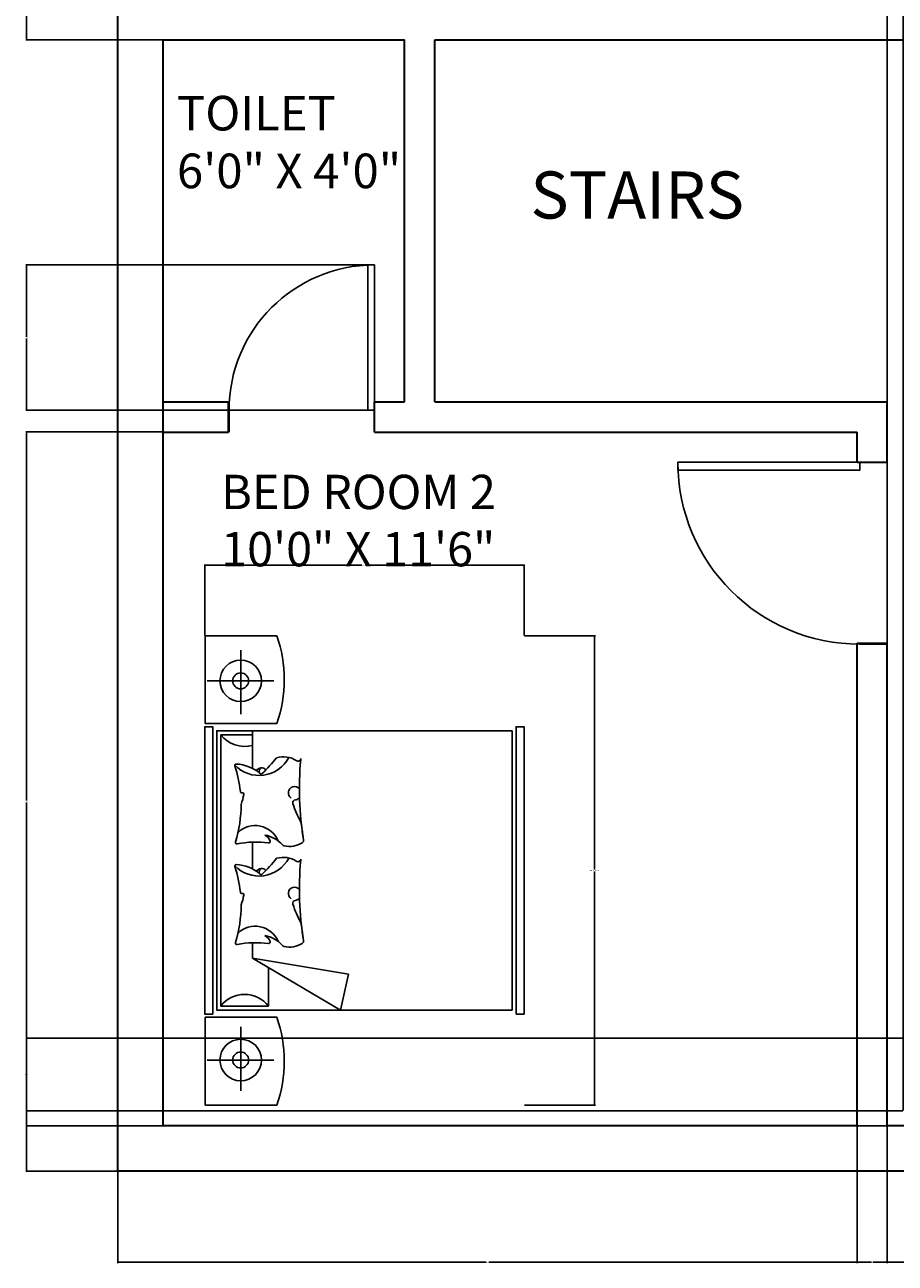
# Model space of a CAD drawing. Units: inches. Extents: x 2360 to 2721, y 1697 to 2094.
# Tile 1 of 3: x 2360 to 2533, y 1697 to 1944. Entities that reach past the tile are written whole.
import ezdxf

# ---------------------------------------------------------------- set-up
doc = ezdxf.new("R2010")
doc.units = ezdxf.units.IN
for name, color, linetype, lineweight in [('A-ANNO-DIMS', 2, 'Continuous', 18), ('A-AREA-IDEN', 7, 'Continuous', 18), ('A-DOOR', 4, 'Continuous', 25), ('A-WALL', 7, 'Continuous', 35), ('FUR', 42, 'Continuous', 18)]:
    doc.layers.add(name, color=color, linetype=linetype, lineweight=lineweight)
for name, color, linetype in [('HID', 11, 'Continuous'), ('SAN', 5, 'Continuous'), ('wood', 26, 'Continuous')]:
    doc.layers.add(name, color=color, linetype=linetype)
doc.styles.get("Standard").update_dxf_attribs({"font": 'arial.ttf'})
doc.dimstyles.get("Standard").update_dxf_attribs({"dimtxt": 0.18, "dimasz": 0.18, "dimexe": 0.18, "dimexo": 0.0625, "dimgap": 0.09, "dimtad": 0, "dimtih": 1, "dimtoh": 1, "dimdec": 4, "dimzin": 0, "dimdsep": 46, "dimtxsty": 'Standard', "dimcen": 0.09, "dimadec": 0, "dimazin": 0, "dimtfac": 1, "dimtdec": 4, "dimtofl": 0, "dimtmove": 0, "dimatfit": 3, "dimfxl": 1, "dimtolj": 1, "dimtzin": 0, "dimarcsym": 0})

# ---------------------------------------------------------------- blocks, each defined once
blk = doc.blocks.new('*U2')
for p, q in [((0, 0), (0, -6)), ((-40, 0), (-40, -6))]:
    blk.add_line(p, q)
blk.add_lwpolyline([(0, 0), (0, 40), (-1.75, 40), (-1.75, 0)], close=True)
blk.add_arc((0, 0), 40, 90, 180)
blk = doc.blocks.new('A$C47AC156F')
at = {"layer": 'HID'}
for centre, radius, start, end in [((1.0153, 1.7986), 0.00933, 72.72477, 190.95899), ((0.3959, 1.6787), 0.6216, 352.73629, 10.95899), ((1.25, 2.5533), 0.781, 252.72477, 270.27016), ((0.9655, 1.684), 0.1552, 292.76276, 43.89219), ((1.25, 2.5533), 0.781, 276.21957, 288.21138), ((1.6451, 1.66), 0.2103, 133.89466, 242.39517), ((1.258, 1.8145), 0.2487, 319.92106, 357.12402), ((1.497, 1.8025), 0.00933, 357.12402, 108.21138), ((1.497, 1.8025), 0.00933, 357.12402, 108.21138), ((1.6455, 1.7986), 0.00933, 72.72477, 190.95899), ((1.0261, 1.6787), 0.6216, 352.73629, 10.95899), ((1.8802, 2.5533), 0.781, 252.72477, 270.27016), ((1.5957, 1.684), 0.1552, 292.76276, 43.89219), ((1.8802, 2.5533), 0.781, 276.21957, 288.21138), ((2.2753, 1.66), 0.2103, 133.89466, 242.39517), ((1.8881, 1.8145), 0.2487, 319.92106, 357.12402), ((2.1272, 1.8025), 0.00933, 357.12402, 108.21138), ((2.1272, 1.8025), 0.00933, 357.12402, 108.21138), ((1.3847, 2.1211), 0.3726, 249.41677, 259.30852), ((1.3173, 1.7641), 0.00933, 259.30852, 10.68903), ((1.3356, 1.7676), 0.00933, 96.21957, 190.68903), ((2.0148, 2.1211), 0.3726, 249.41677, 259.30852), ((1.9474, 1.7641), 0.00933, 259.30852, 10.68903), ((1.9658, 1.7676), 0.00933, 96.21957, 190.68903), ((1.4528, 1.6463), 0.00933, 118.83153, 225.83293), ((2.7269, 2.958), 1.838, 225.83293, 230.02451), ((0.9938, -0.376), 2.0876, 76.49824, 77.28883), ((1.4453, 1.6438), 0.0373, 312.66199, 59.15728), ((2.0829, 1.6463), 0.00933, 118.83153, 225.83293), ((3.357, 2.958), 1.838, 225.83293, 230.02451), ((1.6239, -0.376), 2.0876, 76.49824, 77.28883), ((2.0754, 1.6438), 0.0373, 312.66199, 59.15728), ((0.8707, 1.6576), 0.1939, 311.60711, 349.78448), ((1.0218, 1.5989), 0.00933, 172.73629, 288.29854), ((1.0054, 1.6485), 0.0615, 288.29854, 335.78909), ((0.9938, 3.6438), 2.0876, 282.70178, 282.72062), ((1.5008, 1.6576), 0.1939, 311.60711, 349.78448), ((1.6519, 1.5989), 0.00933, 172.73629, 288.29854), ((1.6355, 1.6485), 0.0615, 288.29854, 335.78909), ((1.6239, 3.6438), 2.0876, 282.70178, 282.72062), ((1.1421, 1.4694), 0.1522, 167.33771, 211.66603), ((1.0118, 1.4987), 0.0187, 131.60711, 167.33771), ((1.3258, 1.4364), 0.0395, 312.35651, 145.77621), ((1.4005, 1.5084), 0.1512, 327.16626, 15.7613), ((1.7723, 1.4694), 0.1522, 167.33771, 211.66603), ((1.642, 1.4987), 0.0187, 131.60711, 167.33771), ((1.9559, 1.4364), 0.0395, 312.35651, 145.77621), ((2.0307, 1.5084), 0.1512, 327.16626, 15.7613), ((1.3501, -0.5337), 1.9409, 84.58522, 99.44651), ((1.1321, 1.4137), 0.0187, 276.38601, 303.79553), ((1.5399, 0.631), 0.864, 109.04896, 117.38232), ((1.264, 1.43), 0.0187, 2.64257, 109.04896), ((1.3013, 1.4318), 0.0187, 182.64257, 192.70152), ((1.3234, 1.4368), 0.0414, 192.70152, 227.15561), ((1.5433, 1.4163), 0.0187, 147.16626, 264.34216), ((1.9802, -0.5337), 1.9409, 84.58522, 99.44651), ((1.7622, 1.4137), 0.0187, 276.38601, 303.79553), ((2.17, 0.631), 0.864, 109.04896, 117.38232), ((1.8941, 1.43), 0.0187, 2.64257, 109.04896), ((1.9314, 1.4318), 0.0187, 182.64257, 192.70152), ((1.9535, 1.4368), 0.0414, 192.70152, 227.15561), ((2.1734, 1.4163), 0.0187, 147.16626, 264.34216), ((1.0285, 1.3993), 0.0187, 211.66603, 279.44651), ((1.3501, -0.5337), 1.9409, 96.38601, 99.44651), ((1.6586, 1.3993), 0.0187, 211.66603, 279.44651), ((1.9802, -0.5337), 1.9409, 96.38601, 99.44651)]:
    blk.add_arc(centre, radius, start, end, dxfattribs=at)
at = {"layer": 'SAN'}
for p, q in [((0.2826, 1.9847), (0.2826, 1.5664)), ((2.6574, 1.9847), (2.6574, 1.5664)), ((0.0902, 1.7748), (0.4911, 1.7748)), ((2.8498, 1.7748), (2.4489, 1.7748))]:
    blk.add_line(p, q, dxfattribs=at)
for centre, radius in [((0.2826, 1.7748), 0.13), ((2.6574, 1.7748), 0.13), ((0.2826, 1.7748), 0.05), ((2.6574, 1.7748), 0.05)]:
    blk.add_circle(centre, radius, dxfattribs=at)
at = {"layer": 'wood'}
for p, q in [((0, 1.9982), (0, 1.5482)), ((0.55, 1.9982), (0, 1.9982)), ((0.55, 1.9982), (0.55, 1.5482)), ((2.39, 1.9982), (2.94, 1.9982)), ((2.39, 1.9982), (2.39, 1.5482)), ((2.94, 1.9982), (2.94, 1.5482)), ((0.62, 1.9), (2.32, 1.9)), ((0.62, 1.9), (0.62, 1.6)), ((2.32, 1.9), (2.32, 1.7)), ((0.92, 1.7), (0.595, 1.15)), ((0.82, 1.1), (0.92, 1.7)), ((1.0171, 1.7), (0.92, 1.7)), ((1.6473, 1.7), (1.4787, 1.7)), ((2.345, 1.7), (2.1088, 1.7)), ((0.62, 1.6), (0.8609, 1.6)), ((0.595, 1.15), (0.82, 1.1))]:
    blk.add_line(p, q, dxfattribs=at)
for points in [[(0.57, 1.95), (2.37, 1.95), (2.37, 2), (0.57, 2)], [(2.345, 0.075), (2.345, 1.925), (0.595, 1.925), (0.595, 0.075)], [(0.57, 0.05), (2.37, 0.05), (2.37, 0), (0.57, 0)]]:
    blk.add_lwpolyline(points, close=True, dxfattribs=at)
for centre, radius, start, end in [((0.5037, 1.75), 0.1898, 307.78263, 52.21737), ((2.4363, 1.75), 0.1898, 127.78263, 195.27469), ((0.275, 2.3419), 0.84, 250.89004, 289.10996), ((2.665, 2.3419), 0.84, 250.89004, 289.10996)]:
    blk.add_arc(centre, radius, start, end, dxfattribs=at)
blk = doc.blocks.new('*D9')
at = {"layer": 'A-ANNO-DIMS', "color": 0, "lineweight": -2, "transparency": 16777216}
for p, q in [((2459.47, 1822.13), (2473.59, 1822.13)), ((2473.41, 1821.95), (2473.41, 1775.63)), ((2473.41, 1728.94), (2473.41, 1775.26)), ((2459.47, 1728.76), (2473.59, 1728.76))]:
    blk.add_line(p, q, dxfattribs=at)
at = {"layer": 'A-ANNO-DIMS', "color": 0, "transparency": 16777216}
for points in [[(2473.38, 1821.95), (2473.44, 1821.95), (2473.41, 1822.13)], [(2473.38, 1728.94), (2473.44, 1728.94), (2473.41, 1728.76)]]:
    blk.add_solid(points, dxfattribs=at)
at = {"layer": 'Defpoints', "color": 0, "transparency": 16777216}
for p in [(2459.41, 1822.13), (2473.41, 1822.13), (2459.41, 1728.76)]:
    blk.add_point(p, dxfattribs=at)
at = {"layer": 'A-ANNO-DIMS', "color": 0, "transparency": 16777216, "insert": (2473.41, 1775.44), "char_height": 0.18, "attachment_point": 5}
blk.add_mtext('\\A1;BED SET 93 TYP.', dxfattribs=at)
blk = doc.blocks.new('*D10')
at = {"layer": 'A-ANNO-DIMS', "color": 0, "lineweight": -2, "transparency": 16777216}
for p, q in [((2395.9, 1822.19), (2395.9, 1836.31)), ((2396.08, 1836.13), (2427.13, 1836.13)), ((2459.23, 1836.13), (2428.18, 1836.13)), ((2459.41, 1822.19), (2459.41, 1836.31))]:
    blk.add_line(p, q, dxfattribs=at)
at = {"layer": 'A-ANNO-DIMS', "color": 0, "transparency": 16777216}
for points in [[(2396.08, 1836.16), (2396.08, 1836.1), (2395.9, 1836.13)], [(2459.23, 1836.16), (2459.23, 1836.1), (2459.41, 1836.13)]]:
    blk.add_solid(points, dxfattribs=at)
at = {"layer": 'Defpoints', "color": 0, "transparency": 16777216}
for p in [(2395.9, 1836.13), (2395.9, 1822.13), (2459.41, 1822.13)]:
    blk.add_point(p, dxfattribs=at)
at = {"layer": 'A-ANNO-DIMS', "color": 0, "transparency": 16777216, "insert": (2427.65, 1836.13), "char_height": 0.18, "attachment_point": 5}
blk.add_mtext('\\A1;64 TYP.', dxfattribs=at)
blk = doc.blocks.new('*D19')
at = {"layer": 'A-ANNO-DIMS', "color": 0, "lineweight": -2, "transparency": 16777216}
for p, q in [((2525.63, 1724.58), (2525.63, 1697.32)), ((2378.63, 1715.58), (2378.63, 1697.32)), ((2378.81, 1697.5), (2451.85, 1697.5)), ((2525.45, 1697.5), (2452.41, 1697.5))]:
    blk.add_line(p, q, dxfattribs=at)
at = {"layer": 'A-ANNO-DIMS', "color": 0, "transparency": 16777216}
for points in [[(2378.81, 1697.53), (2378.81, 1697.47), (2378.63, 1697.5)], [(2525.45, 1697.53), (2525.45, 1697.47), (2525.63, 1697.5)]]:
    blk.add_solid(points, dxfattribs=at)
at = {"layer": 'Defpoints', "color": 0, "transparency": 16777216}
for p in [(2525.63, 1724.65), (2378.63, 1715.65), (2525.63, 1697.5)]:
    blk.add_point(p, dxfattribs=at)
at = {"layer": 'A-ANNO-DIMS', "color": 0, "transparency": 16777216, "insert": (2452.13, 1697.5), "char_height": 0.18, "attachment_point": 5}
blk.add_mtext('\\A1;147', dxfattribs=at)
blk = doc.blocks.new('*D20')
at = {"layer": 'A-ANNO-DIMS', "color": 0, "lineweight": -2, "transparency": 16777216}
for p, q in [((2525.63, 1724.58), (2525.63, 1697.32)), ((2531.63, 1724.58), (2531.63, 1697.32)), ((2525.81, 1697.5), (2528.48, 1697.5)), ((2531.45, 1697.5), (2528.78, 1697.5))]:
    blk.add_line(p, q, dxfattribs=at)
at = {"layer": 'A-ANNO-DIMS', "color": 0, "transparency": 16777216}
for points in [[(2525.81, 1697.53), (2525.81, 1697.47), (2525.63, 1697.5)], [(2531.45, 1697.53), (2531.45, 1697.47), (2531.63, 1697.5)]]:
    blk.add_solid(points, dxfattribs=at)
at = {"layer": 'Defpoints', "color": 0, "transparency": 16777216}
for p in [(2525.63, 1724.65), (2531.63, 1724.65), (2531.63, 1697.5)]:
    blk.add_point(p, dxfattribs=at)
at = {"layer": 'A-ANNO-DIMS', "color": 0, "transparency": 16777216, "insert": (2528.63, 1697.5), "char_height": 0.18, "attachment_point": 5}
blk.add_mtext('\\A1;6', dxfattribs=at)
blk = doc.blocks.new('*D21')
at = {"layer": 'A-ANNO-DIMS', "color": 0, "lineweight": -2, "transparency": 16777216}
for p, q in [((2531.63, 1724.58), (2531.63, 1697.32)), ((2609.63, 1724.58), (2609.63, 1697.32)), ((2531.81, 1697.5), (2570.41, 1697.5)), ((2609.45, 1697.5), (2570.85, 1697.5))]:
    blk.add_line(p, q, dxfattribs=at)
at = {"layer": 'A-ANNO-DIMS', "color": 0, "transparency": 16777216}
for points in [[(2531.81, 1697.53), (2531.81, 1697.47), (2531.63, 1697.5)], [(2609.45, 1697.53), (2609.45, 1697.47), (2609.63, 1697.5)]]:
    blk.add_solid(points, dxfattribs=at)
at = {"layer": 'Defpoints', "color": 0, "transparency": 16777216}
for p in [(2531.63, 1724.65), (2609.63, 1724.65), (2609.63, 1697.5)]:
    blk.add_point(p, dxfattribs=at)
at = {"layer": 'A-ANNO-DIMS', "color": 0, "transparency": 16777216, "insert": (2570.63, 1697.5), "char_height": 0.18, "attachment_point": 5}
blk.add_mtext('\\A1;78', dxfattribs=at)
blk = doc.blocks.new('*D24')
at = {"layer": 'A-ANNO-DIMS', "color": 0, "lineweight": -2, "transparency": 16777216}
for p, q in [((2387.57, 1862.65), (2360.3, 1862.65)), ((2360.48, 1862.47), (2360.48, 1789.33)), ((2360.48, 1715.83), (2360.48, 1788.97)), ((2378.57, 1715.65), (2360.3, 1715.65))]:
    blk.add_line(p, q, dxfattribs=at)
at = {"layer": 'A-ANNO-DIMS', "color": 0, "transparency": 16777216}
for points in [[(2360.45, 1862.47), (2360.51, 1862.47), (2360.48, 1862.65)], [(2360.45, 1715.83), (2360.51, 1715.83), (2360.48, 1715.65)]]:
    blk.add_solid(points, dxfattribs=at)
at = {"layer": 'Defpoints', "color": 0, "transparency": 16777216}
for p in [(2360.48, 1862.65), (2387.63, 1862.65), (2378.63, 1715.65)]:
    blk.add_point(p, dxfattribs=at)
at = {"layer": 'A-ANNO-DIMS', "color": 0, "transparency": 16777216, "insert": (2360.48, 1789.15), "char_height": 0.18, "attachment_point": 5}
blk.add_mtext('\\A1;147', dxfattribs=at)
blk = doc.blocks.new('*D25')
at = {"layer": 'A-ANNO-DIMS', "color": 0, "lineweight": -2, "transparency": 16777216}
for p, q in [((2429.57, 1895.87), (2360.3, 1895.87)), ((2360.48, 1895.69), (2360.48, 1881.61)), ((2360.48, 1867.16), (2360.48, 1881.24)), ((2429.57, 1866.98), (2360.3, 1866.98))]:
    blk.add_line(p, q, dxfattribs=at)
at = {"layer": 'A-ANNO-DIMS', "color": 0, "transparency": 16777216}
for points in [[(2360.45, 1895.69), (2360.51, 1895.69), (2360.48, 1895.87)], [(2360.45, 1867.16), (2360.51, 1867.16), (2360.48, 1866.98)]]:
    blk.add_solid(points, dxfattribs=at)
at = {"layer": 'Defpoints', "color": 0, "transparency": 16777216}
for p in [(2360.48, 1895.87), (2429.63, 1895.87), (2429.63, 1866.98)]:
    blk.add_point(p, dxfattribs=at)
at = {"layer": 'A-ANNO-DIMS', "color": 0, "transparency": 16777216, "insert": (2360.48, 1881.43), "char_height": 0.18, "attachment_point": 5}
blk.add_mtext('\\A1;28.89', dxfattribs=at)
blk = doc.blocks.new('*D26')
at = {"layer": 'A-ANNO-DIMS', "color": 0, "lineweight": -2, "transparency": 16777216}
for p, q in [((2387.57, 1976.65), (2360.3, 1976.65)), ((2360.48, 1976.47), (2360.48, 1958.83)), ((2360.48, 1940.83), (2360.48, 1958.46)), ((2387.57, 1940.65), (2360.3, 1940.65))]:
    blk.add_line(p, q, dxfattribs=at)
at = {"layer": 'A-ANNO-DIMS', "color": 0, "transparency": 16777216}
for points in [[(2360.45, 1976.47), (2360.51, 1976.47), (2360.48, 1976.65)], [(2360.45, 1940.83), (2360.51, 1940.83), (2360.48, 1940.65)]]:
    blk.add_solid(points, dxfattribs=at)
at = {"layer": 'Defpoints', "color": 0, "transparency": 16777216}
for p in [(2360.48, 1976.65), (2387.63, 1976.65), (2387.63, 1940.65)]:
    blk.add_point(p, dxfattribs=at)
at = {"layer": 'A-ANNO-DIMS', "color": 0, "transparency": 16777216, "insert": (2360.48, 1958.65), "char_height": 0.18, "attachment_point": 5}
blk.add_mtext('\\A1;36', dxfattribs=at)
blk = doc.blocks.new('*D36')
at = {"layer": 'A-ANNO-DIMS', "color": 0, "lineweight": -2, "transparency": 16777216}
for p, q in [((2544.4, 1742.08), (2360.3, 1742.08)), ((2360.48, 1741.9), (2360.48, 1735.04)), ((2360.48, 1727.81), (2360.48, 1734.67)), ((2534.77, 1727.63), (2360.3, 1727.63))]:
    blk.add_line(p, q, dxfattribs=at)
at = {"layer": 'A-ANNO-DIMS', "color": 0, "transparency": 16777216}
for points in [[(2360.45, 1741.9), (2360.51, 1741.9), (2360.48, 1742.08)], [(2360.45, 1727.81), (2360.51, 1727.81), (2360.48, 1727.63)]]:
    blk.add_solid(points, dxfattribs=at)
at = {"layer": 'Defpoints', "color": 0, "transparency": 16777216}
for p in [(2360.48, 1742.08), (2544.47, 1742.08), (2534.83, 1727.63)]:
    blk.add_point(p, dxfattribs=at)
at = {"layer": 'A-ANNO-DIMS', "color": 0, "transparency": 16777216, "insert": (2360.48, 1734.85), "char_height": 0.18, "attachment_point": 5}
blk.add_mtext('\\A1;14.454', dxfattribs=at)
blk = doc.blocks.new('*D37')
at = {"layer": 'A-ANNO-DIMS', "color": 0, "lineweight": -2, "transparency": 16777216}
for p, q in [((2531.63, 1724.71), (2531.63, 2093.98)), ((2534.83, 1727.69), (2534.83, 2093.98)), ((2531.81, 2093.8), (2532.84, 2093.8)), ((2534.65, 2093.8), (2533.63, 2093.8))]:
    blk.add_line(p, q, dxfattribs=at)
at = {"layer": 'A-ANNO-DIMS', "color": 0, "transparency": 16777216}
for points in [[(2531.81, 2093.83), (2531.81, 2093.77), (2531.63, 2093.8)], [(2534.65, 2093.83), (2534.65, 2093.77), (2534.83, 2093.8)]]:
    blk.add_solid(points, dxfattribs=at)
at = {"layer": 'Defpoints', "color": 0, "transparency": 16777216}
for p in [(2534.83, 2093.8), (2534.83, 1727.63), (2531.63, 1724.65)]:
    blk.add_point(p, dxfattribs=at)
at = {"layer": 'A-ANNO-DIMS', "color": 0, "transparency": 16777216, "insert": (2533.23, 2093.8), "char_height": 0.18, "attachment_point": 5}
blk.add_mtext('\\A1;3.198', dxfattribs=at)
blk = doc.blocks.new('*D38')
at = {"layer": 'A-ANNO-DIMS', "color": 0, "lineweight": -2, "transparency": 16777216}
for p, q in [((2534.77, 1727.63), (2360.3, 1727.63)), ((2360.48, 1727.45), (2360.48, 1726.32)), ((2531.57, 1724.65), (2360.3, 1724.65)), ((2360.48, 1724.83), (2360.48, 1725.95))]:
    blk.add_line(p, q, dxfattribs=at)
at = {"layer": 'A-ANNO-DIMS', "color": 0, "transparency": 16777216}
for points in [[(2360.45, 1727.45), (2360.51, 1727.45), (2360.48, 1727.63)], [(2360.45, 1724.83), (2360.51, 1724.83), (2360.48, 1724.65)]]:
    blk.add_solid(points, dxfattribs=at)
at = {"layer": 'Defpoints', "color": 0, "transparency": 16777216}
for p in [(2360.48, 1727.63), (2534.83, 1727.63), (2531.63, 1724.65)]:
    blk.add_point(p, dxfattribs=at)
at = {"layer": 'A-ANNO-DIMS', "color": 0, "transparency": 16777216, "insert": (2360.48, 1726.14), "char_height": 0.18, "attachment_point": 5}
blk.add_mtext('\\A1;2.98', dxfattribs=at)

msp = doc.modelspace()

# ---------------------------------------------------------------- linework, layer by layer
at = {"layer": 'A-WALL'}
for p, q in [((2378.6324, 1715.6468), (2378.6324, 2075.6468)), ((2387.6324, 1724.6468), (2387.6324, 1940.6468)), ((2387.6324, 1940.6468), (2435.6324, 1940.6468)), ((2435.6324, 1868.6468), (2435.6324, 1940.6468)), ((2441.6324, 1868.6468), (2441.6324, 1940.6468)), ((2441.6324, 1940.6468), (2561.6324, 1940.6468)), ((2387.6324, 1868.6468), (2400.6324, 1868.6468)), ((2400.6324, 1862.6468), (2400.6324, 1868.6468)), ((2429.6324, 1862.6468), (2429.6324, 1868.6468)), ((2429.6324, 1868.6468), (2435.6324, 1868.6468)), ((2441.6324, 1868.6468), (2531.6324, 1868.6468)), ((2531.6324, 1856.6468), (2531.6324, 1868.6468)), ((2387.6324, 1862.6468), (2400.6324, 1862.6468)), ((2429.6324, 1862.6468), (2525.6324, 1862.6468)), ((2525.6324, 1856.6468), (2525.6324, 1862.6468)), ((2525.6324, 1856.6468), (2531.6324, 1856.6468)), ((2525.6324, 1724.6468), (2525.6324, 1820.6468)), ((2525.6324, 1820.6468), (2531.6324, 1820.6468)), ((2531.6324, 1724.6468), (2531.6324, 1820.6468)), ((2525.6324, 1724.6468), (2387.6324, 1724.6468)), ((2609.6324, 1724.6468), (2531.6324, 1724.6468)), ((2615.6324, 1715.6468), (2378.6324, 1715.6468))]:
    msp.add_line(p, q, dxfattribs=at)

# ---------------------------------------------------------------- block references
at = {"layer": 'A-DOOR', "xscale": 0.7222402786757893, "yscale": 0.7222402786757893, "zscale": 0.7222402786757893}
msp.add_blockref('*U2', (2429.6324, 1866.9802), dxfattribs=at)
at = {"layer": 'A-DOOR', "xscale": 0.9051926542045515, "yscale": 0.9051926542045515, "zscale": 0.9051926542045515, "rotation": 90}
msp.add_blockref('*U2', (2526.2012, 1856.6468), dxfattribs=at)
at = {"layer": 'FUR', "xscale": 31.75566245105898, "yscale": 31.75566245105898, "zscale": 31.75566245105898, "rotation": 90}
msp.add_blockref('A$C47AC156F', (2459.4099, 1728.7639), dxfattribs=at)

# ---------------------------------------------------------------- texts
at = {"layer": 'A-AREA-IDEN', "attachment_point": 1}
for s, width, gutter_width, heights, insert, char_height in [('TOILET\\P6\'0" X 4\'0"', 437.247859, 34.4396, [19.2343], (2390.3789, 1929.5076), 6.88793), ('STAIRS', 594.277356, 46.808, [0], (2460.6793, 1914.4675), 9.3616), ('BED ROOM 2\\P10\'0" X 11\'6"', 433.277752, 34.1269, [0], (2399.1607, 1854.1366), 6.825389)]:
    msp.add_mtext_dynamic_manual_height_columns(s, width=width, gutter_width=gutter_width, heights=heights, dxfattribs=dict(at, insert=insert, char_height=char_height))

# ---------------------------------------------------------------- dimensions: what is measured, and where the dimension line sits
at = {"layer": 'A-ANNO-DIMS'}
for base, p1, p2, override, picture, middle in [((2534.8305, 2093.7968), (2531.6324, 1724.6468), (2534.8305, 1727.6267), {"dimdec": 3, "dimlfac": 1, "dimrnd": 0, "dimzin": 0, "dimdsep": 46, "dimlunit": 2}, '*D37', (2533.2315, 2093.7968)), ((2525.6324, 1697.4968), (2378.6324, 1715.6468), (2525.6324, 1724.6468), {"dimdec": 0, "dimlfac": 1, "dimrnd": 0, "dimzin": 0, "dimdsep": 46, "dimlunit": 2}, '*D19', (2452.1324, 1697.4968)), ((2531.6324, 1697.4968), (2525.6324, 1724.6468), (2531.6324, 1724.6468), {"dimdec": 0, "dimlfac": 1, "dimrnd": 0, "dimzin": 0, "dimdsep": 46, "dimlunit": 2}, '*D20', (2528.6324, 1697.4968)), ((2609.6324, 1697.4968), (2531.6324, 1724.6468), (2609.6324, 1724.6468), {"dimdec": 0, "dimlfac": 1, "dimrnd": 0, "dimzin": 0, "dimdsep": 46, "dimlunit": 2}, '*D21', (2570.6324, 1697.4968))]:
    dim = msp.add_linear_dim(base=base, p1=p1, p2=p2, dimstyle='Standard', override=override, dxfattribs=at)
    dim.commit()
    dim.dimension.update_dxf_attribs({"geometry": picture, "text_midpoint": middle})
for base, p1, p2, override, picture, middle in [((2360.4824, 1976.6468), (2387.6324, 1940.6468), (2387.6324, 1976.6468), {"dimdec": 0, "dimlfac": 1, "dimrnd": 0, "dimzin": 0, "dimdsep": 46, "dimlunit": 2}, '*D26', (2360.4824, 1958.6468)), ((2360.4824, 1895.8698), (2429.6324, 1866.9802), (2429.6324, 1895.8698), {"dimdec": 2, "dimlfac": 1, "dimrnd": 0, "dimzin": 0, "dimdsep": 46, "dimlunit": 2}, '*D25', (2360.4824, 1881.425)), ((2360.4824, 1862.6468), (2378.6324, 1715.6468), (2387.6324, 1862.6468), {"dimdec": 0, "dimlfac": 1, "dimrnd": 0, "dimzin": 0, "dimdsep": 46, "dimlunit": 2}, '*D24', (2360.4824, 1789.1468)), ((2360.4824, 1742.0806), (2534.8305, 1727.6267), (2544.4664, 1742.0806), {"dimdec": 3, "dimlfac": 1, "dimrnd": 0, "dimzin": 0, "dimdsep": 46, "dimlunit": 2}, '*D36', (2360.4824, 1734.8537)), ((2360.4824, 1727.6267), (2531.6324, 1724.6468), (2534.8305, 1727.6267), {"dimdec": 2, "dimlfac": 1, "dimrnd": 0, "dimzin": 0, "dimdsep": 46, "dimlunit": 2}, '*D38', (2360.4824, 1726.1368))]:
    dim = msp.add_linear_dim(base=base, p1=p1, p2=p2, angle=90, dimstyle='Standard', override=override, dxfattribs=at)
    dim.commit()
    dim.dimension.update_dxf_attribs({"geometry": picture, "text_midpoint": middle})
for base, p1, p2, angle, text, picture, middle in [((2395.8986, 1836.1298), (2459.4099, 1822.1255), (2395.8986, 1822.1255), 180, '<> TYP.', '*D10', (2427.6542, 1836.1298)), ((2473.4141, 1822.1255), (2459.4099, 1728.7639), (2459.4099, 1822.1255), 90, 'BED SET <> TYP.', '*D9', (2473.4141, 1775.4447))]:
    dim = msp.add_linear_dim(base=base, p1=p1, p2=p2, angle=angle, text=text, dimstyle='Standard', override={"dimdec": 0, "dimlfac": 1, "dimrnd": 0, "dimzin": 0, "dimdsep": 46, "dimlunit": 2}, dxfattribs=at)
    dim.commit()
    dim.dimension.update_dxf_attribs({"geometry": picture, "text_midpoint": middle})

doc.saveas('drawing.dxf')
